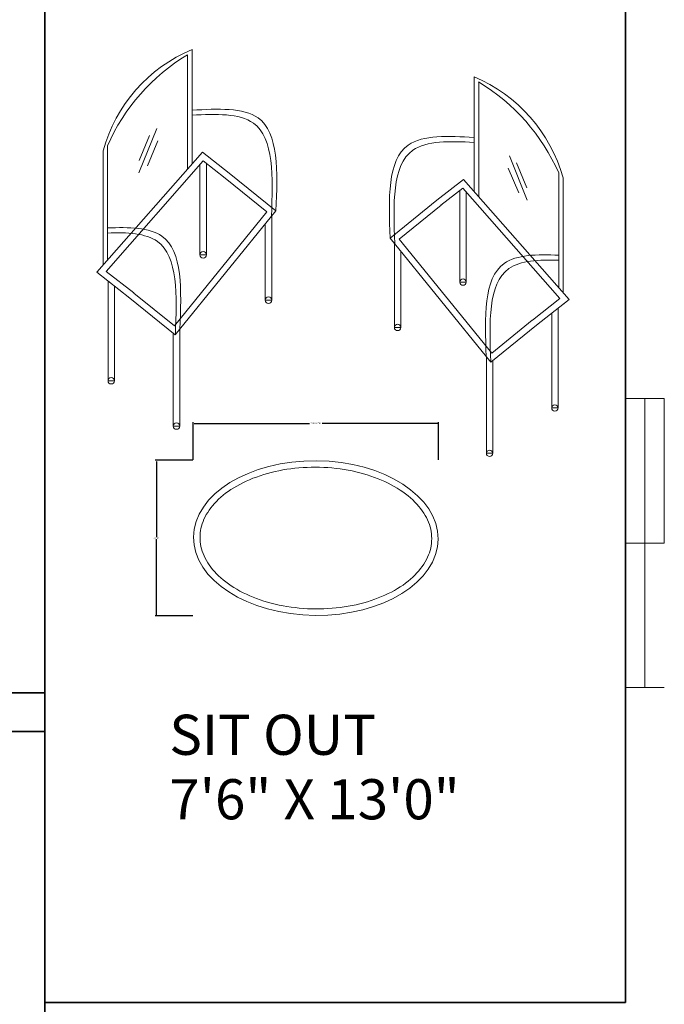
# Model space of a CAD drawing. Units: inches. Extents: x -61 to 1599, y -1316 to 257.
# Tile 162 of 204: x 998 to 1098, y -939 to -787. Entities that reach past the tile are written whole.
import ezdxf

# ---------------------------------------------------------------- set-up
doc = ezdxf.new("R2010")
doc.units = ezdxf.units.IN
doc.header["$MEASUREMENT"] = 0
for name, color, linetype, lineweight in [('A-ANNO-DIMS', 2, 'Continuous', 18), ('A-AREA-IDEN', 1, 'Continuous', 18), ('FURNITURE', 83, 'Continuous', 18), ('WALLS', 4, 'Continuous', 35), ('WINDOWS', 220, 'Continuous', 18)]:
    doc.layers.add(name, color=color, linetype=linetype, lineweight=lineweight)
doc.styles.get("Standard").update_dxf_attribs({"font": 'arial.ttf'})
doc.dimstyles.get("Standard").update_dxf_attribs({"dimtxt": 0.18, "dimasz": 0.18, "dimexe": 0.18, "dimexo": 0.0625, "dimgap": 0.09, "dimtad": 0, "dimtih": 1, "dimtoh": 1, "dimdec": 0, "dimzin": 0, "dimdsep": 46, "dimlunit": 3, "dimtxsty": 'Standard', "dimcen": 0.09, "dimadec": 0, "dimazin": 0, "dimtfac": 1, "dimtdec": 0, "dimtofl": 0, "dimtmove": 0, "dimatfit": 3, "dimfxl": 1, "dimtolj": 1, "dimtzin": 0, "dimarcsym": 0})

# ---------------------------------------------------------------- blocks, each defined once
blk = doc.blocks.new('WIN-45IN')
for p, q in [((0, 44.83), (6, 44.83)), ((0, 0), (6, 0))]:
    blk.add_line(p, q)
for points in [[(6, 44.83), (3, 44.83), (3, 22.42), (6, 22.42)], [(3, 22.42), (0, 22.42), (0, 0), (3, 0)]]:
    blk.add_lwpolyline(points, close=True)
blk = doc.blocks.new('LOUNGE-CHAIR')
for p, q in [((14.04, 40.33), (14.04, 58.08)), ((14.76, 41.14), (14.76, 58.89)), ((6.52, 39.78), (9.29, 46.65)), ((6.58, 41.68), (8.18, 45.54)), ((7.84, 40.87), (9.45, 44.74)), ((0, 24.35), (16.38, 42.98)), ((0.97, 25.45), (0.97, 43.2)), ((0.97, 25.45), (0.97, 43.2)), ((1.64, 26.22), (1.64, 43.97)), ((16.38, 42.98), (20.51, 39.74)), ((1.45, 24.49), (16.5, 41.61)), ((16.5, 41.61), (19.89, 38.96)), ((16.97, 42.52), (16.97, 42.52)), ((16.97, 27.05), (16.97, 41.25)), ((15.97, 27.05), (15.97, 41.01)), ((20.51, 39.74), (27.76, 33.87)), ((19.88, 38.97), (26.35, 33.72)), ((12.02, 16.03), (26.35, 33.72)), ((12.16, 14.63), (27.76, 33.87)), ((27.1, 20.02), (27.1, 33.05)), ((26.1, 20.02), (26.1, 31.82)), ((16.97, 27.05), (15.97, 27.05)), ((1.45, 24.49), (5.72, 21.14)), ((0, 24.35), (5.1, 20.35)), ((0.75, 23.69), (0.79, 23.74)), ((1.73, 7.53), (1.73, 23)), ((2.73, 7.53), (2.73, 22.21)), ((5.1, 20.35), (12.16, 14.63)), ((5.73, 21.13), (12.02, 16.03)), ((27.1, 20.02), (26.1, 20.02)), ((12.85, 0.5), (12.85, 15.48)), ((11.85, 0.5), (11.85, 14.88)), ((2.73, 7.53), (1.73, 7.53)), ((12.85, 0.5), (11.85, 0.5))]:
    blk.add_line(p, q)
for centre in [(16.47, 27.05), (26.6, 20.02), (2.23, 7.53), (12.35, 0.5)]:
    blk.add_circle(centre, 0.5)
for centre, radius, start, end in [((23.93, 36.92), 23.8, 112.6586, 164.6996), ((30.25, 31.33), 31.28, 121.203, 156.1552)]:
    blk.add_arc(centre, radius, start, end)
for points, knots in [([(14.76, 49.49), (18.73, 49.7), (28.38, 50.23), (27.99, 39.93), (27.76, 33.87)], [0, 0, 0, 0, 10.281855, 24.983674, 24.983674, 24.983674, 24.983674]), ([(14.76, 48.72), (18.48, 48.91), (27.65, 49.16), (27.27, 39.12), (27.05, 33.06), (27.04, 33.03), (27.04, 33.01), (27.04, 32.98)], [0.614676, 0.614676, 0.614676, 0.614676, 10.281855, 24.983674, 24.983674, 24.983674, 25.041855, 25.041855, 25.041855, 25.041855]), ([(1.64, 31.22), (4.99, 31.37), (13.47, 31.24), (13.11, 21.57), (12.88, 15.51)], [1.527723, 1.527723, 1.527723, 1.527723, 10.281855, 24.983674, 24.983674, 24.983674, 24.983674]), ([(1.64, 30.44), (4.72, 30.55), (12.75, 30.17), (12.39, 20.76), (12.17, 14.7), (12.16, 14.67), (12.16, 14.65), (12.16, 14.63)], [2.150702, 2.150702, 2.150702, 2.150702, 10.281855, 24.983674, 24.983674, 24.983674, 25.041855, 25.041855, 25.041855, 25.041855])]:
    blk.add_open_spline(points, degree=3, knots=knots)
blk = doc.blocks.new('SIDE-TABLE-OVAL')
blk.add_ellipse((18.95, 11.99), major_axis=(-18.95, 0.16), ratio=0.632617)
blk.add_open_spline([(1, 12.14), (0.99, 11.17), (1.2, 10.2), (2.05, 8.28), (2.69, 7.34), (4.41, 5.58), (5.48, 4.76), (7.96, 3.32), (9.37, 2.71), (12.41, 1.74), (14.05, 1.4), (17.41, 1), (19.13, 0.95), (22.53, 1.15), (24.2, 1.41), (27.36, 2.19), (28.84, 2.73), (31.49, 4.02), (32.66, 4.78), (34.59, 6.45), (35.35, 7.36), (36.44, 9.24), (36.76, 10.2), (36.97, 12.14), (36.87, 13.11), (36.22, 15.04), (35.67, 16), (34.15, 17.81), (33.17, 18.67), (30.85, 20.19), (29.51, 20.86), (26.58, 21.94), (24.98, 22.36), (21.67, 22.89), (19.95, 23.01), (16.54, 22.94), (14.84, 22.76), (11.61, 22.1), (10.07, 21.63), (7.28, 20.44), (6.03, 19.73), (3.92, 18.13), (3.06, 17.25), (1.78, 15.4), (1.35, 14.44), (1.05, 13.03), (1, 12.59), (1, 12.14)], degree=3, knots=[0, 0, 0, 0, 0.279765, 0.279765, 0.559529, 0.559529, 0.839294, 0.839294, 1.119059, 1.119059, 1.398823, 1.398823, 1.678588, 1.678588, 1.958353, 1.958353, 2.238118, 2.238118, 2.517882, 2.517882, 2.797647, 2.797647, 3.077412, 3.077412, 3.357176, 3.357176, 3.636941, 3.636941, 3.916706, 3.916706, 4.19647, 4.19647, 4.476235, 4.476235, 4.756, 4.756, 5.035764, 5.035764, 5.315529, 5.315529, 5.595294, 5.595294, 5.875058, 5.875058, 6.154823, 6.154823, 6.283185, 6.283185, 6.283185, 6.283185])
blk = doc.blocks.new('*D662')
at = {"layer": 'A-ANNO-DIMS', "color": 0, "lineweight": -2, "transparency": 16777216}
for p, q in [((1024.7, -855.01), (1024.7, -849.19)), ((1024.88, -849.37), (1042.75, -849.37)), ((1062.54, -849.37), (1044.68, -849.37)), ((1062.72, -855.01), (1062.72, -849.19))]:
    blk.add_line(p, q, dxfattribs=at)
at = {"layer": 'A-ANNO-DIMS', "color": 0, "transparency": 16777216}
for points in [[(1024.88, -849.34), (1024.88, -849.4), (1024.7, -849.37)], [(1062.54, -849.34), (1062.54, -849.4), (1062.72, -849.37)]]:
    blk.add_solid(points, dxfattribs=at)
at = {"layer": 'DEFPOINTS', "color": 0, "transparency": 16777216}
for p in [(1062.72, -849.37), (1024.7, -855.08), (1062.72, -855.08)]:
    blk.add_point(p, dxfattribs=at)
at = {"layer": 'A-ANNO-DIMS', "color": 0, "transparency": 16777216, "insert": (1043.71, -849.37), "char_height": 0.18, "attachment_point": 5}
blk.add_mtext('\\A1;TABLE 38 TYP.', dxfattribs=at)
blk = doc.blocks.new('*D663')
at = {"layer": 'A-ANNO-DIMS', "color": 0, "lineweight": -2, "transparency": 16777216}
for p, q in [((1024.64, -855.08), (1018.82, -855.08)), ((1019, -855.26), (1019, -866.97)), ((1019, -879.05), (1019, -867.33)), ((1024.64, -879.23), (1018.82, -879.23))]:
    blk.add_line(p, q, dxfattribs=at)
at = {"layer": 'A-ANNO-DIMS', "color": 0, "transparency": 16777216}
for points in [[(1018.97, -855.26), (1019.03, -855.26), (1019, -855.08)], [(1018.97, -879.05), (1019.03, -879.05), (1019, -879.23)]]:
    blk.add_solid(points, dxfattribs=at)
at = {"layer": 'DEFPOINTS', "color": 0, "transparency": 16777216}
for p in [(1019, -855.08), (1024.7, -855.08), (1024.7, -879.23)]:
    blk.add_point(p, dxfattribs=at)
at = {"layer": 'A-ANNO-DIMS', "color": 0, "transparency": 16777216, "insert": (1019, -867.15), "char_height": 0.18, "attachment_point": 5}
blk.add_mtext('\\A1;24 TYP.', dxfattribs=at)

msp = doc.modelspace()

# ---------------------------------------------------------------- linework, layer by layer
at = {"layer": 'WALLS'}
for p, q in [((1001.7028, -1202.169), (1001.7028, -777.169)), ((1091.7028, -939.169), (1091.7028, -783.169)), ((1001.7028, -891.169), (835.7028, -891.169)), ((1001.7028, -897.169), (835.7028, -897.169)), ((1001.7028, -939.169), (1091.7028, -939.169))]:
    msp.add_line(p, q, dxfattribs=at)

# ---------------------------------------------------------------- block references
at = {"layer": 'FURNITURE'}
for name, p in [('LOUNGE-CHAIR', (1009.776, -850.2911)), ('SIDE-TABLE-OVAL', (1024.761, -879.1431))]:
    msp.add_blockref(name, p, dxfattribs=at)
at = {"layer": 'FURNITURE', "extrusion": (0, 0, -1), "zscale": -1}
msp.add_blockref('LOUNGE-CHAIR', (-1082.9843, -854.514), dxfattribs=at)
at = {"layer": 'WINDOWS'}
msp.add_blockref('WIN-45IN', (1091.703, -890.3441), dxfattribs=at)

# ---------------------------------------------------------------- texts
at = {"layer": 'A-AREA-IDEN'}
for s, height, p in [('SIT OUT', 6.22364, (1021.0043, -900.7691)), ('7\'6" X 13\'0"', 6.223643, (1021.0043, -910.7668))]:
    msp.add_text(s, height=height, dxfattribs=at).set_placement(p)

# ---------------------------------------------------------------- dimensions: what is measured, and where the dimension line sits
at = {"layer": 'A-ANNO-DIMS'}
dim = msp.add_linear_dim(base=(1062.7218, -849.3725), p1=(1024.7048, -855.0751), p2=(1062.7218, -855.0751), text='TABLE <> TYP.', dimstyle='Standard', override={"dimdec": 0, "dimlfac": 1, "dimrnd": 0, "dimzin": 0, "dimdsep": 46, "dimlunit": 2}, dxfattribs=at)
dim.commit()
dim.dimension.update_dxf_attribs({"geometry": '*D662', "text_midpoint": (1043.7133, -849.3725)})
dim = msp.add_linear_dim(base=(1019.0022, -855.0751), p1=(1024.7048, -879.2312), p2=(1024.7048, -855.0751), angle=90, text='<> TYP.', dimstyle='Standard', override={"dimdec": 0, "dimlfac": 1, "dimrnd": 0, "dimzin": 0, "dimdsep": 46, "dimlunit": 2}, dxfattribs=at)
dim.commit()
dim.dimension.update_dxf_attribs({"geometry": '*D663', "text_midpoint": (1019.0022, -867.1531)})

doc.saveas('drawing.dxf')
